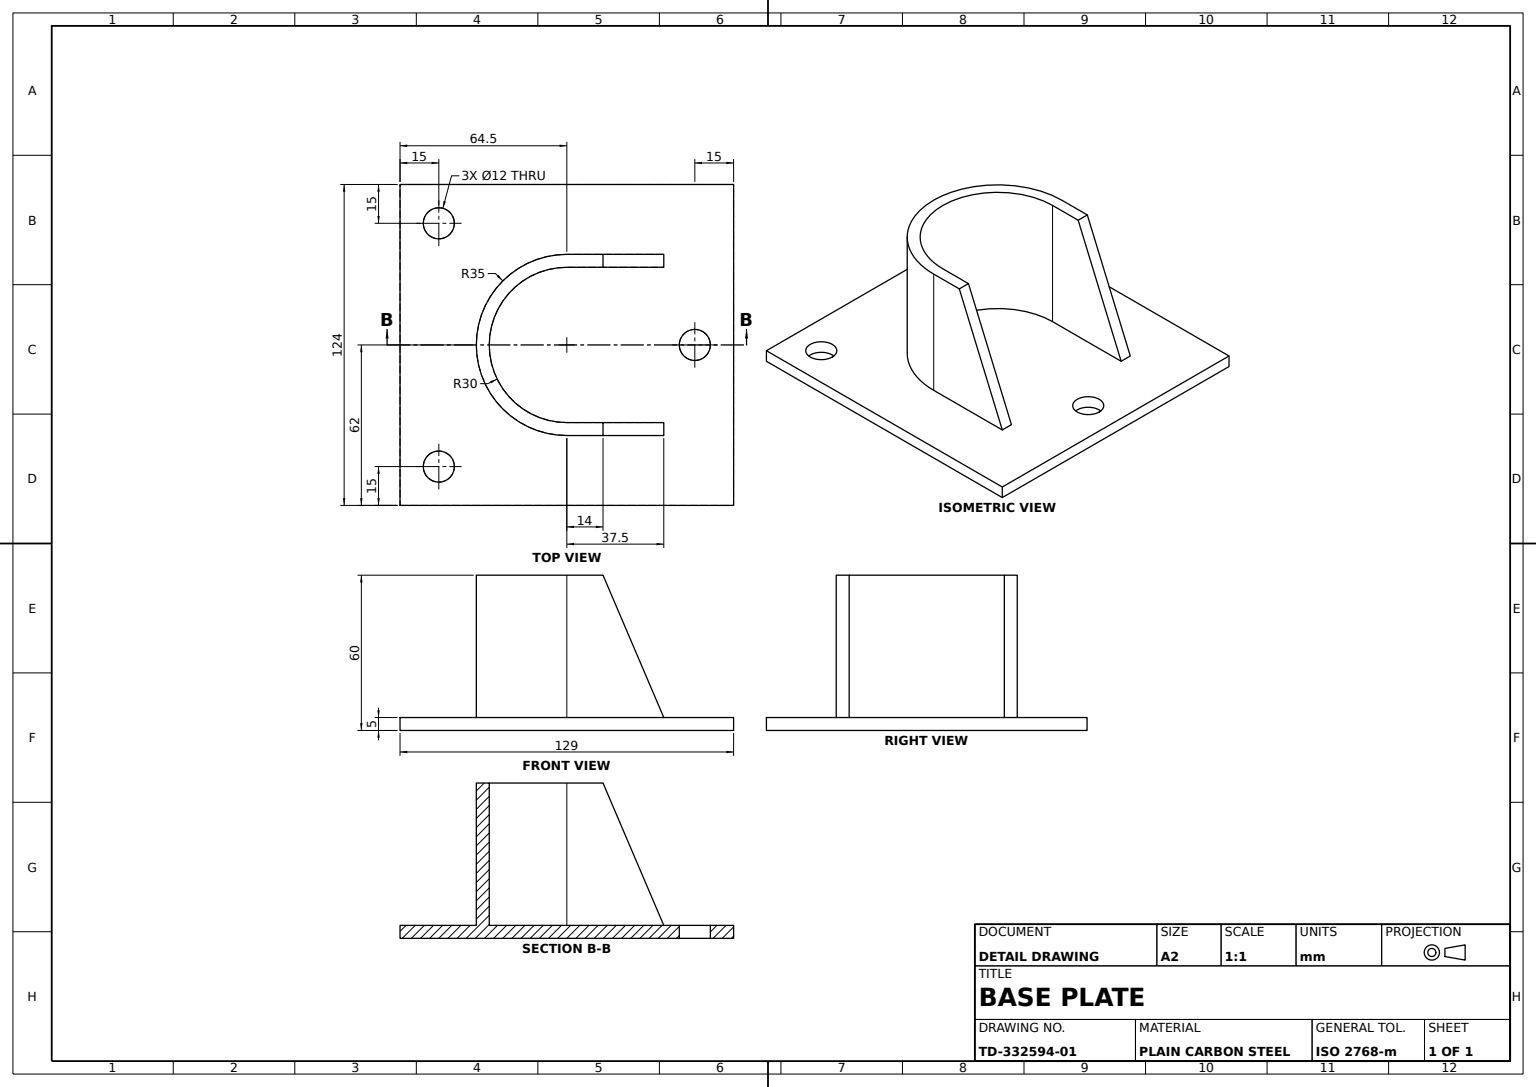
SolidWorks part; units mm, degrees
material "Plain Carbon Steel"
ref_plane "Front Plane" through (0, 0, 0) normal (0, 0, 1) x (1, 0, 0)
ref_plane "Top Plane" through (0, 0, 0) normal (0, 1, 0) x (1, 0, 0)
ref_plane "Right Plane" through (0, 0, 0) normal (1, 0, 0) x (0, 0, -1)
sketch "Base Plate Sketch" plane through (0, 0, 0) normal (0, 1, 0) x (1, 0, 0)
  line L1 (-62, 64.5) -> (62, 64.5)
  line L2 (-62, 64.5) -> (-62, -64.5)
  line L3 (-62, -64.5) -> (62, -64.5)
  line L4 (62, 64.5) -> (62, -64.5)
  line L5 (-62, 64.5) -> (62, -64.5) construction
  line L6 (-62, -64.5) -> (62, 64.5) construction
  circle A0 centre (0, 49.5) radius 6
  circle A1 centre (47, -49.5) radius 6
  circle A2 centre (-47, -49.5) radius 6
  point P0 (0, 0)
  dimension "D2" = 12
  dimension "D3" = 12
  dimension "D9" = 12
  dimension "D1" = 129
  dimension "D4" = 15
  dimension "D5" = 15
  dimension "D6" = 15
  dimension "D7" = 15
  dimension "D8" = 15
  dimension "D10" = 124
extrude "Base Plate" add sketch "Base Plate Sketch" along normal blind 5
sketch "Upright Support Profile Sketch" plane through (0, 0, 0) normal (1, 0, 0) x (0, 0, -1)
  line L0 (37.5, 5) -> (14, 60)
  line L1 (-64.5, 5) -> (64.5, 5) construction
  line L2 (14, 60) -> (-35, 60)
  line L3 (-35, 60) -> (-35, 5)
  line L4 (64.5, 5) -> (64.5, 0) construction
  line L9 (-64.5, 0) -> (64.5, 0)
  line L10 (64.5, 0) -> (64.5, 5)
  line L11 (64.5, 5) -> (-64.5, 5)
  line L12 (-64.5, 5) -> (-64.5, 0)
  line L15 (37.5, 5) -> (-35, 5)
  point P8 (0, 60)
  dimension "D1" = 27
  dimension "D2" = 14
  dimension "D3" = 35
  dimension "D4" = 0
  dimension "D5" = 55
extrude "Upright Support Block" add sketch "Upright Support Profile Sketch" along normal mid plane 70
sketch "Cradle Cut Sketch" plane through (0, 60, 0) normal (0, 1, 0) x (1, 0, 0)
  line L0 (-30, 14) -> (-30, 0)
  line L1 (30, 0) -> (30, 14)
  line L3 (30, 14) -> (30, 37.5)
  line L5 (-30, 37.5) -> (-30, 14)
  line L6 (-35, 14) -> (-35, -35)
  line L7 (-35, -35) -> (35, -35)
  line L8 (35, -35) -> (35, 14)
  line L9 (35, 14) -> (-35, 14)
  line L10 (-35, 14) -> (-35, 0)
  line L12 (35, 0) -> (35, 14)
  line L14 (-35, 37.5) -> (-35, 14)
  line L15 (-35, 14) -> (35, 14)
  line L16 (35, 14) -> (35, 37.5)
  line L17 (35, 37.5) -> (-35, 37.5)
  line L18 (-35, 37.5) -> (-35, 14)
  line L20 (35, 14) -> (35, 37.5)
  line L21 (35, 37.5) -> (30, 37.5)
  line L22 (-30, 32.5) -> (-30, 14) construction
  line L23 (30, 14) -> (30, 32.5) construction
  line L24 (-30, 37.5) -> (-35, 37.5)
  line L25 (35, 37.5) -> (-35, 37.5) construction
  line L26 (30, 32.5) -> (-30, 32.5) construction
  line L27 (35, 37.5) -> (-35, 37.5) construction
  line L28 (35, 37.5) -> (-35, 37.5)
  line L29 (-35, -35) -> (-35, 37.5) construction
  line L30 (-35, -35) -> (-35, 37.5)
  line L31 (35, -35) -> (-35, -35) construction
  line L32 (35, -35) -> (-35, -35)
  line L33 (35, 14) -> (35, -35) construction
  line L34 (35, 14) -> (35, -35)
  arc A0 (-35, 0) -> (35, 0) centre (0, 0) ccw
  arc A1 (-30, 0) -> (30, 0) centre (0, 0) ccw
  line M14 (35, 14) -> (-35, 14)
  dimension "D1" = 5
  dimension "D2" = 70
  dimension "D3" = 0
  dimension "D4" = 0
extrude "Cradle Cut" cut sketch "Cradle Cut Sketch" against normal up to surface (55 mm away) contours L3 L28 L5 M14 | L0 A1 L1 M14 up to face at (47, 5, 55.5)
sketch "Gusset Trim Sketch" plane through (0, 60, 0) normal (0, 1, 0) x (1, 0, 0)
  line L0 (35, 14) -> (35, -35) construction
  line L1 (35, -35) -> (-35, -35) construction
  line L2 (-35, -35) -> (-35, 37.5) construction
  line L3 (35, 0) -> (35, -35)
  line L4 (35, -35) -> (-35, -35)
  line L5 (-35, -35) -> (-35, 0)
  arc A0 (-35, 0) -> (35, 0) centre (0, 0) ccw construction
  arc A1 (-35, 0) -> (35, 0) centre (0, 0) ccw
  line M6 (-35, 14) -> (-35, -35)
  line M7 (-35, -35) -> (35, -35)
  line M8 (35, -35) -> (35, 14)
extrude "Gusset Trim Cut" cut sketch "Gusset Trim Sketch" along direction (0, 1, 0) on the side against the normal blind 55 contours A1 M6 M7 | A1 L4 M8
